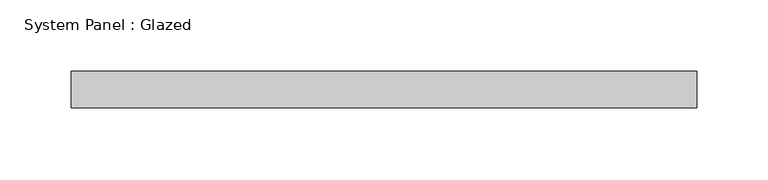
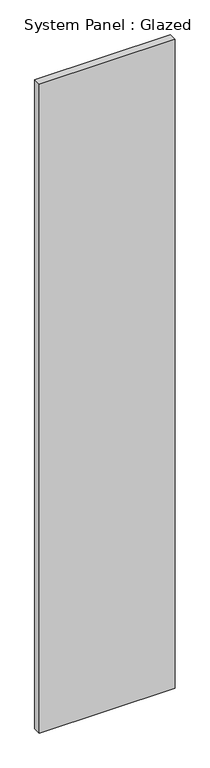
"""IFC4 building model written with IfcOpenShell, lengths in millimetres: plate geometry, System Panel : Glazed."""

from ifc_helpers import new_model, si_unit, origin, origin_with_axes, place, context, project, spatial, polyline, outline, extrude, source, transform, mapped, element, save


def system_panel_glazed_6abed3b5(model_context):
    return source(origin(), model_context, "Body", "SweptSolid", [
        extrude(outline(polyline([(219.075, 19.05), (-219.075, 19.05), (-219.075, 44.45), (219.075, 44.45), (219.075, 19.05)])), origin_with_axes(), (0.0, 0.0, 1.0), 2209.8),
    ])


if __name__ == "__main__":
    model = new_model("IFC4")
    model_context = context("Model", 3, world=origin())
    ifc_project = project(units=[si_unit("LENGTHUNIT", "METRE", prefix="MILLI")], contexts=[model_context])
    site = spatial("IfcSite", under=ifc_project)
    building = spatial("IfcBuilding", under=site)
    placement = place(None, origin())
    system_panel_glazed_shape = system_panel_glazed_6abed3b5(model_context)
    element("IfcPlate", 1, ObjectType="System Panel : Glazed", at=placement, inside=building, context=model_context, shape_type="MappedRepresentation", body=[
        mapped(system_panel_glazed_shape, transform((0.0, 0.0, 0.0), x_axis=(1.0, 0.0, 0.0), y_axis=(0.0, 1.0, 0.0), z_axis=(0.0, 0.0, 1.0))),
    ])
    save(model, "model.ifc")

# Revit data of these elements
# Type "System Panel : Glazed"
#   Construction Type Id = "GSP4R"
#   Analytic Construction = "1/8 in Pilkington single glazing"
#   Visual Light Transmittance = 0.9
#   Solar Heat Gain Coefficient = 0.86
#   Heat Transfer Coefficient (U) = 1.18115 BTU/(h·ft²·°F)
#   Define Thermal Properties by = 1
# Element 1 (IfcPlate, "System Panel : Glazed")
#   Materials on its faces: "Glass"
# Materials
#   "Glass": class "Glass", colour RGB 0 128 192, transparency 0.75, Description = "Soda Lime Glass", Cost = 0
